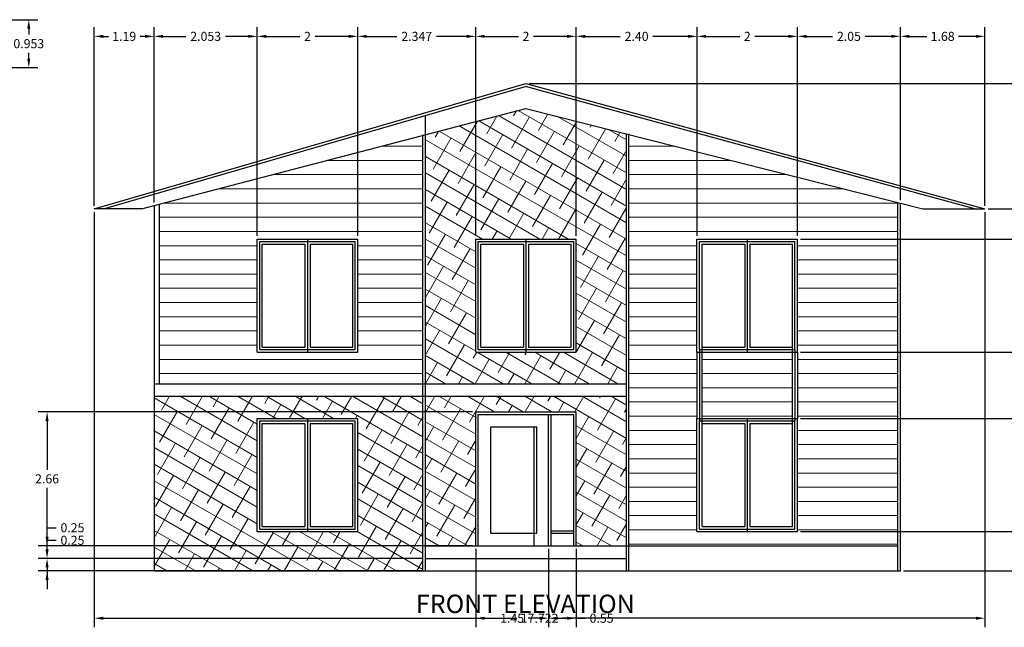
# Model space of a CAD drawing. Units: metres. Extents: x 14054 to 28215, y 4175 to 8383.
# Tile 4 of 6: x 14077.36 to 14096.96, y 4179.61 to 4191.69. Entities that reach past the tile are written whole.
import ezdxf

# ---------------------------------------------------------------- set-up
doc = ezdxf.new("R2010")
doc.units = ezdxf.units.M
for name, color, linetype, lineweight in [('A-ANNO-DIMS', 2, 'Continuous', 18), ('A-ANNO-TEXT', 3, 'Continuous', 18), ('A-ELEV', 7, 'Continuous', 25), ('A-WALL-PATT', 8, 'Continuous', 13)]:
    doc.layers.add(name, color=color, linetype=linetype, lineweight=lineweight)
doc.styles.get("Standard").update_dxf_attribs({"font": 'arial.ttf'})
doc.dimstyles.get("Standard").update_dxf_attribs({"dimtxt": 0.18, "dimasz": 0.18, "dimexe": 0.18, "dimexo": 0.0625, "dimgap": 0.09, "dimtad": 0, "dimtih": 1, "dimtoh": 1, "dimdec": 4, "dimzin": 0, "dimdsep": 46, "dimtxsty": 'Standard', "dimcen": 0.09, "dimadec": 0, "dimazin": 0, "dimtfac": 1, "dimtdec": 4, "dimtofl": 0, "dimtmove": 0, "dimatfit": 3, "dimfxl": 1, "dimtolj": 1, "dimtzin": 0, "dimarcsym": 0})

# ---------------------------------------------------------------- blocks, each defined once
blk = doc.blocks.new('*D13')
at = {"layer": 'A-ANNO-DIMS', "color": 0, "lineweight": -2, "transparency": 16777216}
for p, q in [((14078.849, 4187.865), (14078.849, 4179.608)), ((14096.571, 4187.865), (14096.571, 4179.608)), ((14079.029, 4179.788), (14087.256, 4179.788)), ((14096.391, 4179.788), (14088.164, 4179.788))]:
    blk.add_line(p, q, dxfattribs=at)
at = {"layer": 'A-ANNO-DIMS', "color": 0, "transparency": 16777216}
for points in [[(14079.029, 4179.818), (14079.029, 4179.758), (14078.849, 4179.788)], [(14096.391, 4179.818), (14096.391, 4179.758), (14096.571, 4179.788)]]:
    blk.add_solid(points, dxfattribs=at)
at = {"layer": 'Defpoints', "color": 0, "transparency": 16777216}
for p in [(14078.849, 4187.928), (14096.571, 4187.928), (14096.571, 4179.788)]:
    blk.add_point(p, dxfattribs=at)
at = {"layer": 'A-ANNO-DIMS', "color": 0, "transparency": 16777216, "insert": (14087.71, 4179.788), "char_height": 0.18, "attachment_point": 5}
blk.add_mtext('\\A1;17.722', dxfattribs=at)
blk = doc.blocks.new('*D14')
at = {"layer": 'A-ANNO-DIMS', "color": 0, "lineweight": -2, "transparency": 16777216}
for p, q in [((14078.849, 4187.99), (14078.849, 4191.54)), ((14080.038, 4188.055), (14080.038, 4191.54)), ((14079.029, 4191.36), (14079.128, 4191.36)), ((14079.858, 4191.36), (14079.759, 4191.36))]:
    blk.add_line(p, q, dxfattribs=at)
at = {"layer": 'A-ANNO-DIMS', "color": 0, "transparency": 16777216}
for points in [[(14079.029, 4191.39), (14079.029, 4191.33), (14078.849, 4191.36)], [(14079.858, 4191.39), (14079.858, 4191.33), (14080.038, 4191.36)]]:
    blk.add_solid(points, dxfattribs=at)
at = {"layer": 'Defpoints', "color": 0, "transparency": 16777216}
for p in [(14080.038, 4191.36), (14078.849, 4187.928), (14080.038, 4187.993)]:
    blk.add_point(p, dxfattribs=at)
at = {"layer": 'A-ANNO-DIMS', "color": 0, "transparency": 16777216, "insert": (14079.444, 4191.36), "char_height": 0.18, "attachment_point": 5}
blk.add_mtext('\\A1;1.19', dxfattribs=at)
blk = doc.blocks.new('*D15')
at = {"layer": 'A-ANNO-DIMS', "color": 0, "lineweight": -2, "transparency": 16777216}
for p, q in [((14080.038, 4188.055), (14080.038, 4191.54)), ((14082.091, 4187.392), (14082.091, 4191.54)), ((14080.218, 4191.36), (14080.669, 4191.36)), ((14081.911, 4191.36), (14081.46, 4191.36))]:
    blk.add_line(p, q, dxfattribs=at)
at = {"layer": 'A-ANNO-DIMS', "color": 0, "transparency": 16777216}
for points in [[(14080.218, 4191.39), (14080.218, 4191.33), (14080.038, 4191.36)], [(14081.911, 4191.39), (14081.911, 4191.33), (14082.091, 4191.36)]]:
    blk.add_solid(points, dxfattribs=at)
at = {"layer": 'Defpoints', "color": 0, "transparency": 16777216}
for p in [(14082.091, 4191.36), (14080.038, 4187.993), (14082.091, 4187.329)]:
    blk.add_point(p, dxfattribs=at)
at = {"layer": 'A-ANNO-DIMS', "color": 0, "transparency": 16777216, "insert": (14081.065, 4191.36), "char_height": 0.18, "attachment_point": 5}
blk.add_mtext('\\A1;2.053', dxfattribs=at)
blk = doc.blocks.new('*D16')
at = {"layer": 'A-ANNO-DIMS', "color": 0, "lineweight": -2, "transparency": 16777216}
for p, q in [((14082.091, 4187.392), (14082.091, 4191.54)), ((14084.091, 4187.392), (14084.091, 4191.54)), ((14082.271, 4191.36), (14082.941, 4191.36)), ((14083.911, 4191.36), (14083.241, 4191.36))]:
    blk.add_line(p, q, dxfattribs=at)
at = {"layer": 'A-ANNO-DIMS', "color": 0, "transparency": 16777216}
for points in [[(14082.271, 4191.39), (14082.271, 4191.33), (14082.091, 4191.36)], [(14083.911, 4191.39), (14083.911, 4191.33), (14084.091, 4191.36)]]:
    blk.add_solid(points, dxfattribs=at)
at = {"layer": 'Defpoints', "color": 0, "transparency": 16777216}
for p in [(14084.091, 4191.36), (14082.091, 4187.329), (14084.091, 4187.329)]:
    blk.add_point(p, dxfattribs=at)
at = {"layer": 'A-ANNO-DIMS', "color": 0, "transparency": 16777216, "insert": (14083.091, 4191.36), "char_height": 0.18, "attachment_point": 5}
blk.add_mtext('\\A1;2', dxfattribs=at)
blk = doc.blocks.new('*D17')
at = {"layer": 'A-ANNO-DIMS', "color": 0, "lineweight": -2, "transparency": 16777216}
for p, q in [((14084.091, 4187.392), (14084.091, 4191.54)), ((14086.438, 4187.392), (14086.438, 4191.54)), ((14084.271, 4191.36), (14084.869, 4191.36)), ((14086.258, 4191.36), (14085.66, 4191.36))]:
    blk.add_line(p, q, dxfattribs=at)
at = {"layer": 'A-ANNO-DIMS', "color": 0, "transparency": 16777216}
for points in [[(14084.271, 4191.39), (14084.271, 4191.33), (14084.091, 4191.36)], [(14086.258, 4191.39), (14086.258, 4191.33), (14086.438, 4191.36)]]:
    blk.add_solid(points, dxfattribs=at)
at = {"layer": 'Defpoints', "color": 0, "transparency": 16777216}
for p in [(14086.438, 4191.36), (14084.091, 4187.329), (14086.438, 4187.329)]:
    blk.add_point(p, dxfattribs=at)
at = {"layer": 'A-ANNO-DIMS', "color": 0, "transparency": 16777216, "insert": (14085.265, 4191.36), "char_height": 0.18, "attachment_point": 5}
blk.add_mtext('\\A1;2.347', dxfattribs=at)
blk = doc.blocks.new('*D18')
at = {"layer": 'A-ANNO-DIMS', "color": 0, "lineweight": -2, "transparency": 16777216}
for p, q in [((14086.438, 4187.392), (14086.438, 4191.54)), ((14088.438, 4187.392), (14088.438, 4191.54)), ((14086.618, 4191.36), (14087.289, 4191.36)), ((14088.258, 4191.36), (14087.588, 4191.36))]:
    blk.add_line(p, q, dxfattribs=at)
at = {"layer": 'A-ANNO-DIMS', "color": 0, "transparency": 16777216}
for points in [[(14086.618, 4191.39), (14086.618, 4191.33), (14086.438, 4191.36)], [(14088.258, 4191.39), (14088.258, 4191.33), (14088.438, 4191.36)]]:
    blk.add_solid(points, dxfattribs=at)
at = {"layer": 'Defpoints', "color": 0, "transparency": 16777216}
for p in [(14088.438, 4191.36), (14086.438, 4187.329), (14088.438, 4187.329)]:
    blk.add_point(p, dxfattribs=at)
at = {"layer": 'A-ANNO-DIMS', "color": 0, "transparency": 16777216, "insert": (14087.438, 4191.36), "char_height": 0.18, "attachment_point": 5}
blk.add_mtext('\\A1;2', dxfattribs=at)
blk = doc.blocks.new('*D19')
at = {"layer": 'A-ANNO-DIMS', "color": 0, "lineweight": -2, "transparency": 16777216}
for p, q in [((14088.438, 4187.392), (14088.438, 4191.54)), ((14090.842, 4187.392), (14090.842, 4191.54)), ((14088.618, 4191.36), (14089.315, 4191.36)), ((14090.662, 4191.36), (14089.965, 4191.36))]:
    blk.add_line(p, q, dxfattribs=at)
at = {"layer": 'A-ANNO-DIMS', "color": 0, "transparency": 16777216}
for points in [[(14088.618, 4191.39), (14088.618, 4191.33), (14088.438, 4191.36)], [(14090.662, 4191.39), (14090.662, 4191.33), (14090.842, 4191.36)]]:
    blk.add_solid(points, dxfattribs=at)
at = {"layer": 'Defpoints', "color": 0, "transparency": 16777216}
for p in [(14090.842, 4191.36), (14088.438, 4187.329), (14090.842, 4187.329)]:
    blk.add_point(p, dxfattribs=at)
at = {"layer": 'A-ANNO-DIMS', "color": 0, "transparency": 16777216, "insert": (14089.64, 4191.36), "char_height": 0.18, "attachment_point": 5}
blk.add_mtext('\\A1;2.40', dxfattribs=at)
blk = doc.blocks.new('*D20')
at = {"layer": 'A-ANNO-DIMS', "color": 0, "lineweight": -2, "transparency": 16777216}
for p, q in [((14090.842, 4187.392), (14090.842, 4191.54)), ((14092.842, 4187.392), (14092.842, 4191.54)), ((14091.022, 4191.36), (14091.692, 4191.36)), ((14092.662, 4191.36), (14091.991, 4191.36))]:
    blk.add_line(p, q, dxfattribs=at)
at = {"layer": 'A-ANNO-DIMS', "color": 0, "transparency": 16777216}
for points in [[(14091.022, 4191.39), (14091.022, 4191.33), (14090.842, 4191.36)], [(14092.662, 4191.39), (14092.662, 4191.33), (14092.842, 4191.36)]]:
    blk.add_solid(points, dxfattribs=at)
at = {"layer": 'Defpoints', "color": 0, "transparency": 16777216}
for p in [(14092.842, 4191.36), (14090.842, 4187.329), (14092.842, 4187.329)]:
    blk.add_point(p, dxfattribs=at)
at = {"layer": 'A-ANNO-DIMS', "color": 0, "transparency": 16777216, "insert": (14091.842, 4191.36), "char_height": 0.18, "attachment_point": 5}
blk.add_mtext('\\A1;2', dxfattribs=at)
blk = doc.blocks.new('*D21')
at = {"layer": 'A-ANNO-DIMS', "color": 0, "lineweight": -2, "transparency": 16777216}
for p, q in [((14092.842, 4187.392), (14092.842, 4191.54)), ((14094.888, 4188.104), (14094.888, 4191.54)), ((14093.022, 4191.36), (14093.539, 4191.36)), ((14094.708, 4191.36), (14094.191, 4191.36))]:
    blk.add_line(p, q, dxfattribs=at)
at = {"layer": 'A-ANNO-DIMS', "color": 0, "transparency": 16777216}
for points in [[(14093.022, 4191.39), (14093.022, 4191.33), (14092.842, 4191.36)], [(14094.708, 4191.39), (14094.708, 4191.33), (14094.888, 4191.36)]]:
    blk.add_solid(points, dxfattribs=at)
at = {"layer": 'Defpoints', "color": 0, "transparency": 16777216}
for p in [(14094.888, 4191.36), (14094.888, 4188.041), (14092.842, 4187.329)]:
    blk.add_point(p, dxfattribs=at)
at = {"layer": 'A-ANNO-DIMS', "color": 0, "transparency": 16777216, "insert": (14093.865, 4191.36), "char_height": 0.18, "attachment_point": 5}
blk.add_mtext('\\A1;2.05', dxfattribs=at)
blk = doc.blocks.new('*D22')
at = {"layer": 'A-ANNO-DIMS', "color": 0, "lineweight": -2, "transparency": 16777216}
for p, q in [((14094.888, 4188.104), (14094.888, 4191.54)), ((14096.571, 4187.99), (14096.571, 4191.54)), ((14095.068, 4191.36), (14095.414, 4191.36)), ((14096.391, 4191.36), (14096.045, 4191.36))]:
    blk.add_line(p, q, dxfattribs=at)
at = {"layer": 'A-ANNO-DIMS', "color": 0, "transparency": 16777216}
for points in [[(14095.068, 4191.39), (14095.068, 4191.33), (14094.888, 4191.36)], [(14096.391, 4191.39), (14096.391, 4191.33), (14096.571, 4191.36)]]:
    blk.add_solid(points, dxfattribs=at)
at = {"layer": 'Defpoints', "color": 0, "transparency": 16777216}
for p in [(14096.571, 4191.36), (14094.888, 4188.041), (14096.571, 4187.928)]:
    blk.add_point(p, dxfattribs=at)
at = {"layer": 'A-ANNO-DIMS', "color": 0, "transparency": 16777216, "insert": (14095.73, 4191.36), "char_height": 0.18, "attachment_point": 5}
blk.add_mtext('\\A1;1.68', dxfattribs=at)
blk = doc.blocks.new('*D23')
at = {"layer": 'A-ANNO-DIMS', "color": 0, "lineweight": -2, "transparency": 16777216}
for p, q in [((14097.511, 4181.511), (14097.511, 4181.691)), ((14097.511, 4181.691), (14097.691, 4181.691)), ((14092.904, 4181.511), (14097.691, 4181.511)), ((14097.511, 4180.908), (14097.511, 4181.331)), ((14094.951, 4180.728), (14097.691, 4180.728))]:
    blk.add_line(p, q, dxfattribs=at)
at = {"layer": 'A-ANNO-DIMS', "color": 0, "transparency": 16777216}
for points in [[(14097.481, 4181.331), (14097.541, 4181.331), (14097.511, 4181.511)], [(14097.481, 4180.908), (14097.541, 4180.908), (14097.511, 4180.728)]]:
    blk.add_solid(points, dxfattribs=at)
at = {"layer": 'Defpoints', "color": 0, "transparency": 16777216}
for p in [(14092.842, 4181.511), (14097.511, 4181.511), (14094.888, 4180.728)]:
    blk.add_point(p, dxfattribs=at)
at = {"layer": 'A-ANNO-DIMS', "color": 0, "transparency": 16777216, "insert": (14098.084, 4181.691), "char_height": 0.18, "attachment_point": 5}
blk.add_mtext('\\A1;0.784', dxfattribs=at)
blk = doc.blocks.new('*D24')
at = {"layer": 'A-ANNO-DIMS', "color": 0, "lineweight": -2, "transparency": 16777216}
for p, q in [((14092.904, 4183.761), (14097.691, 4183.761)), ((14097.511, 4183.581), (14097.511, 4182.818)), ((14097.511, 4181.691), (14097.511, 4182.454)), ((14092.904, 4181.511), (14097.691, 4181.511))]:
    blk.add_line(p, q, dxfattribs=at)
at = {"layer": 'A-ANNO-DIMS', "color": 0, "transparency": 16777216}
for points in [[(14097.481, 4183.581), (14097.541, 4183.581), (14097.511, 4183.761)], [(14097.481, 4181.691), (14097.541, 4181.691), (14097.511, 4181.511)]]:
    blk.add_solid(points, dxfattribs=at)
at = {"layer": 'Defpoints', "color": 0, "transparency": 16777216}
for p in [(14092.842, 4183.761), (14097.511, 4183.761), (14092.842, 4181.511)]:
    blk.add_point(p, dxfattribs=at)
at = {"layer": 'A-ANNO-DIMS', "color": 0, "transparency": 16777216, "insert": (14097.511, 4182.636), "char_height": 0.18, "attachment_point": 5}
blk.add_mtext('\\A1;2.25', dxfattribs=at)
blk = doc.blocks.new('*D25')
at = {"layer": 'A-ANNO-DIMS', "color": 0, "lineweight": -2, "transparency": 16777216}
for p, q in [((14092.904, 4185.079), (14097.691, 4185.079)), ((14097.511, 4184.899), (14097.511, 4184.602)), ((14097.511, 4183.941), (14097.511, 4184.238)), ((14092.904, 4183.761), (14097.691, 4183.761))]:
    blk.add_line(p, q, dxfattribs=at)
at = {"layer": 'A-ANNO-DIMS', "color": 0, "transparency": 16777216}
for points in [[(14097.481, 4184.899), (14097.541, 4184.899), (14097.511, 4185.079)], [(14097.481, 4183.941), (14097.541, 4183.941), (14097.511, 4183.761)]]:
    blk.add_solid(points, dxfattribs=at)
at = {"layer": 'Defpoints', "color": 0, "transparency": 16777216}
for p in [(14092.842, 4185.079), (14097.511, 4185.079), (14092.842, 4183.761)]:
    blk.add_point(p, dxfattribs=at)
at = {"layer": 'A-ANNO-DIMS', "color": 0, "transparency": 16777216, "insert": (14097.511, 4184.42), "char_height": 0.18, "attachment_point": 5}
blk.add_mtext('\\A1;1.318', dxfattribs=at)
blk = doc.blocks.new('*D26')
at = {"layer": 'A-ANNO-DIMS', "color": 0, "lineweight": -2, "transparency": 16777216}
for p, q in [((14092.904, 4187.329), (14097.691, 4187.329)), ((14097.511, 4187.149), (14097.511, 4186.386)), ((14097.511, 4185.259), (14097.511, 4186.022)), ((14092.904, 4185.079), (14097.691, 4185.079))]:
    blk.add_line(p, q, dxfattribs=at)
at = {"layer": 'A-ANNO-DIMS', "color": 0, "transparency": 16777216}
for points in [[(14097.481, 4187.149), (14097.541, 4187.149), (14097.511, 4187.329)], [(14097.481, 4185.259), (14097.541, 4185.259), (14097.511, 4185.079)]]:
    blk.add_solid(points, dxfattribs=at)
at = {"layer": 'Defpoints', "color": 0, "transparency": 16777216}
for p in [(14092.842, 4187.329), (14097.511, 4187.329), (14092.842, 4185.079)]:
    blk.add_point(p, dxfattribs=at)
at = {"layer": 'A-ANNO-DIMS', "color": 0, "transparency": 16777216, "insert": (14097.511, 4186.204), "char_height": 0.18, "attachment_point": 5}
blk.add_mtext('\\A1;2.25', dxfattribs=at)
blk = doc.blocks.new('*D27')
at = {"layer": 'A-ANNO-DIMS', "color": 0, "lineweight": -2, "transparency": 16777216}
for p, q in [((14097.511, 4187.928), (14097.511, 4188.108)), ((14097.511, 4188.108), (14097.691, 4188.108)), ((14096.633, 4187.928), (14097.691, 4187.928)), ((14097.511, 4187.509), (14097.511, 4187.748)), ((14092.904, 4187.329), (14097.691, 4187.329))]:
    blk.add_line(p, q, dxfattribs=at)
at = {"layer": 'A-ANNO-DIMS', "color": 0, "transparency": 16777216}
for points in [[(14097.481, 4187.748), (14097.541, 4187.748), (14097.511, 4187.928)], [(14097.481, 4187.509), (14097.541, 4187.509), (14097.511, 4187.329)]]:
    blk.add_solid(points, dxfattribs=at)
at = {"layer": 'Defpoints', "color": 0, "transparency": 16777216}
for p in [(14096.571, 4187.928), (14097.511, 4187.928), (14092.842, 4187.329)]:
    blk.add_point(p, dxfattribs=at)
at = {"layer": 'A-ANNO-DIMS', "color": 0, "transparency": 16777216, "insert": (14098.014, 4188.108), "char_height": 0.18, "attachment_point": 5}
blk.add_mtext('\\A1;0.60', dxfattribs=at)
blk = doc.blocks.new('*D28')
at = {"layer": 'A-ANNO-DIMS', "color": 0, "lineweight": -2, "transparency": 16777216}
for p, q in [((14087.501, 4190.42), (14097.691, 4190.42)), ((14097.511, 4190.24), (14097.511, 4189.356)), ((14097.511, 4188.108), (14097.511, 4188.992)), ((14096.633, 4187.928), (14097.691, 4187.928))]:
    blk.add_line(p, q, dxfattribs=at)
at = {"layer": 'A-ANNO-DIMS', "color": 0, "transparency": 16777216}
for points in [[(14097.481, 4190.24), (14097.541, 4190.24), (14097.511, 4190.42)], [(14097.481, 4188.108), (14097.541, 4188.108), (14097.511, 4187.928)]]:
    blk.add_solid(points, dxfattribs=at)
at = {"layer": 'Defpoints', "color": 0, "transparency": 16777216}
for p in [(14087.438, 4190.42), (14097.511, 4190.42), (14096.571, 4187.928)]:
    blk.add_point(p, dxfattribs=at)
at = {"layer": 'A-ANNO-DIMS', "color": 0, "transparency": 16777216, "insert": (14097.511, 4189.174), "char_height": 0.18, "attachment_point": 5}
blk.add_mtext('\\A1;2.49', dxfattribs=at)
blk = doc.blocks.new('*D40')
at = {"layer": 'A-ANNO-DIMS', "color": 0, "lineweight": -2, "transparency": 16777216}
for p, q in [((14086.438, 4181.165), (14086.438, 4179.608)), ((14087.888, 4181.165), (14087.888, 4179.608)), ((14086.618, 4179.788), (14086.847, 4179.788)), ((14087.708, 4179.788), (14087.479, 4179.788))]:
    blk.add_line(p, q, dxfattribs=at)
at = {"layer": 'A-ANNO-DIMS', "color": 0, "transparency": 16777216}
for points in [[(14086.618, 4179.818), (14086.618, 4179.758), (14086.438, 4179.788)], [(14087.708, 4179.818), (14087.708, 4179.758), (14087.888, 4179.788)]]:
    blk.add_solid(points, dxfattribs=at)
at = {"layer": 'Defpoints', "color": 0, "transparency": 16777216}
for p in [(14086.438, 4181.228), (14087.888, 4181.228), (14087.888, 4179.788)]:
    blk.add_point(p, dxfattribs=at)
at = {"layer": 'A-ANNO-DIMS', "color": 0, "transparency": 16777216, "insert": (14087.163, 4179.788), "char_height": 0.18, "attachment_point": 5}
blk.add_mtext('\\A1;1.45', dxfattribs=at)
blk = doc.blocks.new('*D41')
at = {"layer": 'A-ANNO-DIMS', "color": 0, "lineweight": -2, "transparency": 16777216}
for p, q in [((14087.888, 4181.165), (14087.888, 4179.608)), ((14088.438, 4181.165), (14088.438, 4179.608)), ((14088.068, 4179.788), (14088.258, 4179.788)), ((14088.438, 4179.788), (14088.618, 4179.788))]:
    blk.add_line(p, q, dxfattribs=at)
at = {"layer": 'A-ANNO-DIMS', "color": 0, "transparency": 16777216}
for points in [[(14088.068, 4179.818), (14088.068, 4179.758), (14087.888, 4179.788)], [(14088.258, 4179.818), (14088.258, 4179.758), (14088.438, 4179.788)]]:
    blk.add_solid(points, dxfattribs=at)
at = {"layer": 'Defpoints', "color": 0, "transparency": 16777216}
for p in [(14087.888, 4181.228), (14088.438, 4181.228), (14088.438, 4179.788)]:
    blk.add_point(p, dxfattribs=at)
at = {"layer": 'A-ANNO-DIMS', "color": 0, "transparency": 16777216, "insert": (14088.943, 4179.788), "char_height": 0.18, "attachment_point": 5}
blk.add_mtext('\\A1;0.55', dxfattribs=at)
blk = doc.blocks.new('*D42')
at = {"layer": 'A-ANNO-DIMS', "color": 0, "lineweight": -2, "transparency": 16777216}
for p, q in [((14086.376, 4183.892), (14077.729, 4183.892)), ((14077.909, 4183.712), (14077.909, 4182.742)), ((14077.909, 4181.408), (14077.909, 4182.378)), ((14086.376, 4181.228), (14077.729, 4181.228))]:
    blk.add_line(p, q, dxfattribs=at)
at = {"layer": 'A-ANNO-DIMS', "color": 0, "transparency": 16777216}
for points in [[(14077.879, 4183.712), (14077.939, 4183.712), (14077.909, 4183.892)], [(14077.879, 4181.408), (14077.939, 4181.408), (14077.909, 4181.228)]]:
    blk.add_solid(points, dxfattribs=at)
at = {"layer": 'Defpoints', "color": 0, "transparency": 16777216}
for p in [(14077.909, 4183.892), (14086.438, 4183.892), (14086.438, 4181.228)]:
    blk.add_point(p, dxfattribs=at)
at = {"layer": 'A-ANNO-DIMS', "color": 0, "transparency": 16777216, "insert": (14077.909, 4182.56), "char_height": 0.18, "attachment_point": 5}
blk.add_mtext('\\A1;2.66', dxfattribs=at)
blk = doc.blocks.new('*D43')
at = {"layer": 'A-ANNO-DIMS', "color": 0, "lineweight": -2, "transparency": 16777216}
for p, q in [((14077.909, 4181.158), (14077.909, 4181.338)), ((14077.909, 4181.338), (14078.089, 4181.338)), ((14085.376, 4180.978), (14077.729, 4180.978)), ((14085.376, 4180.728), (14077.729, 4180.728)), ((14077.909, 4180.548), (14077.909, 4180.368))]:
    blk.add_line(p, q, dxfattribs=at)
at = {"layer": 'A-ANNO-DIMS', "color": 0, "transparency": 16777216}
for points in [[(14077.879, 4181.158), (14077.939, 4181.158), (14077.909, 4180.978)], [(14077.879, 4180.548), (14077.939, 4180.548), (14077.909, 4180.728)]]:
    blk.add_solid(points, dxfattribs=at)
at = {"layer": 'Defpoints', "color": 0, "transparency": 16777216}
for p in [(14077.909, 4180.978), (14085.438, 4180.978), (14085.438, 4180.728)]:
    blk.add_point(p, dxfattribs=at)
at = {"layer": 'A-ANNO-DIMS', "color": 0, "transparency": 16777216, "insert": (14078.414, 4181.338), "char_height": 0.18, "attachment_point": 5}
blk.add_mtext('\\A1;0.25', dxfattribs=at)
blk = doc.blocks.new('*D44')
at = {"layer": 'A-ANNO-DIMS', "color": 0, "lineweight": -2, "transparency": 16777216}
for p, q in [((14077.909, 4181.408), (14077.909, 4181.588)), ((14077.909, 4181.588), (14078.089, 4181.588)), ((14085.376, 4181.228), (14077.729, 4181.228)), ((14085.376, 4180.978), (14077.729, 4180.978)), ((14077.909, 4180.798), (14077.909, 4180.618))]:
    blk.add_line(p, q, dxfattribs=at)
at = {"layer": 'A-ANNO-DIMS', "color": 0, "transparency": 16777216}
for points in [[(14077.879, 4181.408), (14077.939, 4181.408), (14077.909, 4181.228)], [(14077.879, 4180.798), (14077.939, 4180.798), (14077.909, 4180.978)]]:
    blk.add_solid(points, dxfattribs=at)
at = {"layer": 'Defpoints', "color": 0, "transparency": 16777216}
for p in [(14077.909, 4181.228), (14085.438, 4181.228), (14085.438, 4180.978)]:
    blk.add_point(p, dxfattribs=at)
at = {"layer": 'A-ANNO-DIMS', "color": 0, "transparency": 16777216, "insert": (14078.414, 4181.588), "char_height": 0.18, "attachment_point": 5}
blk.add_mtext('\\A1;0.25', dxfattribs=at)
blk = doc.blocks.new('*D75')
at = {"layer": 'A-ANNO-DIMS', "color": 0, "lineweight": -2, "transparency": 16777216}
for p, q in [((14073.161, 4191.691), (14077.725, 4191.691)), ((14077.545, 4191.511), (14077.545, 4191.397)), ((14077.545, 4190.918), (14077.545, 4191.033)), ((14073.161, 4190.738), (14077.725, 4190.738))]:
    blk.add_line(p, q, dxfattribs=at)
at = {"layer": 'A-ANNO-DIMS', "color": 0, "transparency": 16777216}
for points in [[(14077.515, 4191.511), (14077.575, 4191.511), (14077.545, 4191.691)], [(14077.515, 4190.918), (14077.575, 4190.918), (14077.545, 4190.738)]]:
    blk.add_solid(points, dxfattribs=at)
at = {"layer": 'Defpoints', "color": 0, "transparency": 16777216}
for p in [(14073.099, 4191.691), (14073.099, 4190.738), (14077.545, 4190.738)]:
    blk.add_point(p, dxfattribs=at)
at = {"layer": 'A-ANNO-DIMS', "color": 0, "transparency": 16777216, "insert": (14077.545, 4191.215), "char_height": 0.18, "attachment_point": 5}
blk.add_mtext('\\A1;0.953', dxfattribs=at)

msp = doc.modelspace()

# ---------------------------------------------------------------- hatches: boundary and pattern name
at = {"layer": 'A-WALL-PATT'}
h = msp.add_hatch(dxfattribs=at)
h.set_pattern_fill('ANSI38', color=256, scale=0.09, angle=105)
h.paths.add_polyline_path([(14085.3882, 4184.2025), (14080.0382, 4184.2025), (14080.0382, 4180.7275), (14085.3882, 4180.7275)])
h.paths.add_polyline_path([(14084.091, 4183.7614), (14084.091, 4181.5114), (14082.091, 4181.5114), (14082.091, 4183.7614)], flags=16)
h.paths.add_polyline_path([(14084.041, 4183.7114), (14084.041, 4181.5614), (14082.141, 4181.5614), (14082.141, 4183.7114)], flags=0)
h.paths.add_polyline_path([(14083.991, 4183.6614), (14083.991, 4181.6114), (14083.141, 4181.6114), (14083.141, 4183.6614)], flags=0)
h.paths.add_polyline_path([(14083.041, 4183.6614), (14083.041, 4181.6114), (14082.191, 4181.6114), (14082.191, 4183.6614)], flags=0)
h.paths.add_polyline_path([(14086.4382, 4183.892), (14088.4382, 4183.892), (14088.4382, 4181.2275), (14089.4382, 4181.2275), (14089.4382, 4184.2025), (14085.4382, 4184.2025), (14085.4382, 4181.2275), (14086.4382, 4181.2275)])
h.paths.add_polyline_path([(14089.4382, 4189.4203), (14087.4382, 4189.9263), (14085.4382, 4189.4038), (14085.4382, 4184.4525), (14089.4382, 4184.4525)])
h.paths.add_polyline_path([(14086.4382, 4187.3294), (14088.4382, 4187.3294), (14088.4382, 4185.0794), (14086.4382, 4185.0794)], flags=16)
h.paths.add_polyline_path([(14086.4882, 4187.2794), (14088.3882, 4187.2794), (14088.3882, 4185.1294), (14086.4882, 4185.1294)], flags=0)
h.paths.add_polyline_path([(14086.5382, 4187.2294), (14087.3882, 4187.2294), (14087.3882, 4185.1794), (14086.5382, 4185.1794)], flags=0)
h.paths.add_polyline_path([(14087.4882, 4187.2294), (14088.3382, 4187.2294), (14088.3382, 4185.1794), (14087.4882, 4185.1794)], flags=0)
h = msp.add_hatch(dxfattribs=at)
h.set_pattern_fill('ANSI31', color=256, scale=0.089, angle=135)
h.paths.add_polyline_path([(14085.3882, 4189.3907), (14080.1382, 4188.019), (14080.1382, 4184.4525), (14085.3882, 4184.4525)])
h.paths.add_polyline_path([(14084.091, 4187.3294), (14084.091, 4185.0794), (14082.091, 4185.0794), (14082.091, 4187.3294)], flags=16)
h.paths.add_polyline_path([(14084.041, 4187.2794), (14084.041, 4185.1294), (14082.141, 4185.1294), (14082.141, 4187.2794)], flags=0)
h.paths.add_polyline_path([(14083.991, 4187.2294), (14083.991, 4185.1794), (14083.141, 4185.1794), (14083.141, 4187.2294)], flags=0)
h.paths.add_polyline_path([(14083.041, 4187.2294), (14083.041, 4185.1794), (14082.191, 4185.1794), (14082.191, 4187.2294)], flags=0)
h = msp.add_hatch(dxfattribs=at)
h.set_pattern_fill('ANSI31', color=256, scale=0.089, angle=135)
h.paths.add_polyline_path([(14094.8382, 4188.054), (14089.4882, 4189.4077), (14089.4882, 4181.2275), (14094.8382, 4181.2275)])
h.paths.add_polyline_path([(14090.8417, 4187.3294), (14092.8417, 4187.3294), (14092.8417, 4185.0794), (14092.8417, 4183.7614), (14092.8417, 4181.5114), (14090.8417, 4181.5114), (14090.8417, 4183.7614), (14090.8417, 4185.0794)], flags=16)
h.paths.add_polyline_path([(14090.8917, 4187.2794), (14092.7917, 4187.2794), (14092.7917, 4185.1294), (14092.7917, 4183.7114), (14092.7917, 4181.5614), (14090.8917, 4181.5614), (14090.8917, 4183.7114), (14090.8917, 4185.1294)], flags=0)
h.paths.add_polyline_path([(14090.9417, 4187.2294), (14091.7917, 4187.2294), (14091.7917, 4185.1794), (14090.9417, 4185.1794), (14090.9417, 4185.1294), (14092.7417, 4185.1294), (14092.7417, 4185.1794), (14091.8917, 4185.1794), (14091.8917, 4187.2294), (14092.7417, 4187.2294), (14092.7417, 4185.1794), (14092.7417, 4183.6614), (14092.7417, 4181.6114), (14091.8917, 4181.6114), (14091.8917, 4183.6614), (14092.7417, 4183.6614), (14092.7417, 4183.7114), (14090.9417, 4183.7114), (14090.9417, 4183.6614), (14091.7917, 4183.6614), (14091.7917, 4181.6114), (14090.9417, 4181.6114), (14090.9417, 4183.6614), (14090.9417, 4185.1794)], flags=0)
h = msp.add_hatch(dxfattribs=at)
h.set_pattern_fill('ANSI31', color=256, scale=0.089, angle=135)
h.paths.add_polyline_path([(14092.7417, 4185.0794), (14090.9417, 4185.0794), (14090.9417, 4183.7614), (14092.7417, 4183.7614)])

# ---------------------------------------------------------------- linework, layer by layer
at = {"layer": 'A-ELEV'}
for p, q in [((14078.8491, 4187.9275), (14087.4382, 4190.4202)), ((14079.0285, 4187.9275), (14087.4522, 4190.3722)), ((14087.425, 4190.372), (14096.3811, 4187.9275)), ((14087.4382, 4190.4202), (14096.571, 4187.9275)), ((14079.7882, 4187.9275), (14087.4382, 4189.9263)), ((14085.4382, 4184.2025), (14085.4382, 4189.7877)), ((14087.4382, 4189.9263), (14095.3382, 4187.9275)), ((14085.3882, 4184.2025), (14085.3882, 4189.4038)), ((14089.4382, 4180.7275), (14089.4382, 4189.4203)), ((14089.4882, 4180.7275), (14089.4882, 4189.4203)), ((14080.1382, 4188.019), (14080.1382, 4184.4525)), ((14094.8382, 4180.7275), (14094.8382, 4188.054)), ((14094.8882, 4180.7275), (14094.8882, 4188.0414)), ((14079.7882, 4187.9275), (14078.8491, 4187.9275)), ((14080.0382, 4187.9928), (14080.0382, 4180.7275)), ((14095.3382, 4187.9275), (14096.571, 4187.9275)), ((14082.091, 4185.0794), (14082.091, 4187.3294)), ((14082.091, 4187.3294), (14084.091, 4187.3294)), ((14082.141, 4187.2794), (14084.041, 4187.2794)), ((14082.141, 4185.1294), (14082.141, 4187.2794)), ((14082.191, 4187.2294), (14083.041, 4187.2294)), ((14082.191, 4185.1794), (14082.191, 4187.2294)), ((14083.041, 4187.2294), (14083.041, 4185.1794)), ((14083.091, 4187.3294), (14083.091, 4185.0794)), ((14083.141, 4187.2294), (14083.991, 4187.2294)), ((14083.141, 4187.2294), (14083.141, 4185.1794)), ((14083.991, 4185.1794), (14083.991, 4187.2294)), ((14084.041, 4185.1294), (14084.041, 4187.2794)), ((14084.091, 4185.0794), (14084.091, 4187.3294)), ((14086.4382, 4185.0794), (14086.4382, 4187.3294)), ((14086.4382, 4187.3294), (14088.4382, 4187.3294)), ((14086.4882, 4185.1294), (14086.4882, 4187.2794)), ((14086.4882, 4187.2794), (14088.3882, 4187.2794)), ((14086.5382, 4185.1794), (14086.5382, 4187.2294)), ((14086.5382, 4187.2294), (14087.3882, 4187.2294)), ((14087.3882, 4187.2294), (14087.3882, 4185.1794)), ((14087.4382, 4187.3294), (14087.4382, 4185.0794)), ((14087.4882, 4187.2294), (14088.3382, 4187.2294)), ((14087.4882, 4187.2294), (14087.4882, 4185.1794)), ((14088.3382, 4185.1794), (14088.3382, 4187.2294)), ((14088.3882, 4185.1294), (14088.3882, 4187.2794)), ((14088.4382, 4185.0794), (14088.4382, 4187.3294)), ((14090.8417, 4185.0794), (14090.8417, 4187.3294)), ((14090.8417, 4187.3294), (14092.8417, 4187.3294)), ((14090.8917, 4185.1294), (14090.8917, 4187.2794)), ((14090.8917, 4187.2794), (14092.7917, 4187.2794)), ((14090.9417, 4185.1794), (14090.9417, 4187.2294)), ((14090.9417, 4187.2294), (14091.7917, 4187.2294)), ((14091.7917, 4187.2294), (14091.7917, 4185.1794)), ((14091.8417, 4187.3294), (14091.8417, 4185.0794)), ((14091.8917, 4187.2294), (14092.7417, 4187.2294)), ((14091.8917, 4187.2294), (14091.8917, 4185.1794)), ((14092.7417, 4185.1794), (14092.7417, 4187.2294)), ((14092.7917, 4185.1294), (14092.7917, 4187.2794)), ((14092.8417, 4185.0794), (14092.8417, 4187.3294)), ((14082.091, 4185.0794), (14084.091, 4185.0794)), ((14082.141, 4185.1294), (14084.041, 4185.1294)), ((14082.191, 4185.1794), (14083.041, 4185.1794)), ((14083.141, 4185.1794), (14083.991, 4185.1794)), ((14086.4382, 4185.0794), (14088.4382, 4185.0794)), ((14086.4882, 4185.1294), (14088.3882, 4185.1294)), ((14086.5382, 4185.1794), (14087.3882, 4185.1794)), ((14087.4882, 4185.1794), (14088.3382, 4185.1794)), ((14090.8417, 4185.0794), (14092.8417, 4185.0794)), ((14090.8417, 4185.0794), (14090.8417, 4183.7614)), ((14090.8917, 4185.1294), (14092.7917, 4185.1294)), ((14090.8917, 4185.1294), (14090.8917, 4183.7114)), ((14090.9417, 4185.1794), (14091.7917, 4185.1794)), ((14090.9417, 4183.6614), (14090.9417, 4185.1794)), ((14091.8917, 4185.1794), (14092.7417, 4185.1794)), ((14092.7417, 4183.6614), (14092.7417, 4185.1794)), ((14092.7917, 4185.1294), (14092.7917, 4183.7114)), ((14092.8417, 4185.0794), (14092.8417, 4183.7614)), ((14080.0382, 4184.4525), (14089.4382, 4184.4525)), ((14080.0382, 4184.2025), (14089.4382, 4184.2025)), ((14085.3882, 4180.7275), (14085.3882, 4184.2025)), ((14085.4382, 4180.7275), (14085.4382, 4184.2025)), ((14086.4382, 4181.2275), (14086.4382, 4183.892)), ((14086.4382, 4183.892), (14088.4382, 4183.892)), ((14088.4382, 4181.2275), (14088.4382, 4183.892)), ((14082.091, 4181.5114), (14082.091, 4183.7614)), ((14082.091, 4183.7614), (14084.091, 4183.7614)), ((14082.141, 4181.5614), (14082.141, 4183.7114)), ((14082.141, 4183.7114), (14084.041, 4183.7114)), ((14083.091, 4183.7614), (14083.091, 4181.5114)), ((14084.041, 4181.5614), (14084.041, 4183.7114)), ((14084.091, 4181.5114), (14084.091, 4183.7614)), ((14086.4882, 4181.2275), (14086.4882, 4183.842)), ((14086.4882, 4183.842), (14088.3882, 4183.842)), ((14087.8882, 4181.2275), (14087.8882, 4183.842)), ((14087.9382, 4181.2275), (14087.9382, 4183.842)), ((14088.3882, 4181.2275), (14088.3882, 4183.842)), ((14090.8417, 4181.5114), (14090.8417, 4183.7614)), ((14090.8417, 4183.7614), (14092.8417, 4183.7614)), ((14090.8917, 4181.5614), (14090.8917, 4183.7114)), ((14090.8917, 4183.7114), (14092.7917, 4183.7114)), ((14091.8417, 4183.7614), (14091.8417, 4181.5114)), ((14092.7917, 4181.5614), (14092.7917, 4183.7114)), ((14092.8417, 4181.5114), (14092.8417, 4183.7614)), ((14082.191, 4181.6114), (14082.191, 4183.6614)), ((14082.191, 4183.6614), (14083.041, 4183.6614)), ((14083.041, 4183.6614), (14083.041, 4181.6114)), ((14083.141, 4183.6614), (14083.991, 4183.6614)), ((14083.141, 4183.6614), (14083.141, 4181.6114)), ((14083.991, 4181.6114), (14083.991, 4183.6614)), ((14086.7382, 4183.592), (14087.6522, 4183.592)), ((14086.7382, 4181.4775), (14086.7382, 4183.592)), ((14087.6022, 4181.2275), (14087.6022, 4183.592)), ((14087.6522, 4181.4775), (14087.6522, 4183.592)), ((14090.9417, 4181.6114), (14090.9417, 4183.6614)), ((14090.9417, 4183.6614), (14091.7917, 4183.6614)), ((14091.7917, 4183.6614), (14091.7917, 4181.6114)), ((14091.8917, 4183.6614), (14092.7417, 4183.6614)), ((14091.8917, 4183.6614), (14091.8917, 4181.6114)), ((14092.7417, 4181.6114), (14092.7417, 4183.6614)), ((14082.141, 4181.5614), (14084.041, 4181.5614)), ((14082.191, 4181.6114), (14083.041, 4181.6114)), ((14083.141, 4181.6114), (14083.991, 4181.6114)), ((14090.8917, 4181.5614), (14092.7917, 4181.5614)), ((14090.9417, 4181.6114), (14091.7917, 4181.6114)), ((14091.8917, 4181.6114), (14092.7417, 4181.6114)), ((14082.091, 4181.5114), (14084.091, 4181.5114)), ((14086.7382, 4181.4775), (14087.6522, 4181.4775)), ((14087.9382, 4181.5275), (14088.3882, 4181.5275)), ((14087.9382, 4181.4775), (14088.3882, 4181.4775)), ((14090.8417, 4181.5114), (14092.8417, 4181.5114)), ((14085.4382, 4181.2275), (14089.4382, 4181.2275)), ((14087.9382, 4181.2275), (14088.3882, 4181.2275)), ((14089.4382, 4181.2275), (14094.8382, 4181.2275)), ((14085.4382, 4180.9775), (14089.4382, 4180.9775)), ((14080.0382, 4180.7275), (14094.8882, 4180.7275))]:
    msp.add_line(p, q, dxfattribs=at)

# ---------------------------------------------------------------- texts
at = {"layer": 'A-ANNO-TEXT'}
msp.add_text('FRONT ELEVATION', height=0.365459, dxfattribs=at).set_placement((14085.2483, 4179.8912))

# ---------------------------------------------------------------- dimensions: what is measured, and where the dimension line sits
at = {"layer": 'A-ANNO-DIMS'}
for base, p1, p2, override, picture, middle in [((14077.5449, 4190.7382), (14073.099, 4191.6913), (14073.099, 4190.7382), {"dimdec": 3, "dimlfac": 1, "dimrnd": 0, "dimzin": 0, "dimdsep": 46, "dimlunit": 2}, '*D75', (14077.5449, 4191.2147)), ((14097.511, 4190.4202), (14096.571, 4187.9275), (14087.4382, 4190.4202), {"dimdec": 2, "dimlfac": 1, "dimrnd": 0, "dimzin": 0, "dimdsep": 46, "dimlunit": 2}, '*D28', (14097.511, 4189.1739)), ((14097.511, 4187.9275), (14092.8417, 4187.3294), (14096.571, 4187.9275), {"dimdec": 2, "dimlfac": 1, "dimrnd": 0, "dimzin": 0, "dimdsep": 46, "dimlunit": 2}, '*D27', (14098.0145, 4188.1075)), ((14097.511, 4187.3294), (14092.8417, 4185.0794), (14092.8417, 4187.3294), {"dimdec": 2, "dimlfac": 1, "dimrnd": 0, "dimzin": 0, "dimdsep": 46, "dimlunit": 2}, '*D26', (14097.511, 4186.2044)), ((14097.511, 4185.0794), (14092.8417, 4183.7614), (14092.8417, 4185.0794), {"dimdec": 3, "dimlfac": 1, "dimrnd": 0, "dimzin": 0, "dimdsep": 46, "dimlunit": 2}, '*D25', (14097.511, 4184.4204)), ((14077.9091, 4183.892), (14086.4382, 4181.2275), (14086.4382, 4183.892), {"dimdec": 2, "dimlfac": 1, "dimrnd": 0, "dimzin": 0, "dimdsep": 46, "dimlunit": 2}, '*D42', (14077.9091, 4182.5598)), ((14097.511, 4183.7614), (14092.8417, 4181.5114), (14092.8417, 4183.7614), {"dimdec": 2, "dimlfac": 1, "dimrnd": 0, "dimzin": 0, "dimdsep": 46, "dimlunit": 2}, '*D24', (14097.511, 4182.6364)), ((14097.511, 4181.5114), (14094.8882, 4180.7275), (14092.8417, 4181.5114), {"dimdec": 3, "dimlfac": 1, "dimrnd": 0, "dimzin": 0, "dimdsep": 46, "dimlunit": 2}, '*D23', (14098.0843, 4181.6914)), ((14077.9091, 4181.2275), (14085.4382, 4180.9775), (14085.4382, 4181.2275), {"dimdec": 2, "dimlfac": 1, "dimrnd": 0, "dimzin": 0, "dimdsep": 46, "dimlunit": 2}, '*D44', (14078.4135, 4181.5875)), ((14077.9091, 4180.9775), (14085.4382, 4180.7275), (14085.4382, 4180.9775), {"dimdec": 2, "dimlfac": 1, "dimrnd": 0, "dimzin": 0, "dimdsep": 46, "dimlunit": 2}, '*D43', (14078.4135, 4181.3375))]:
    dim = msp.add_linear_dim(base=base, p1=p1, p2=p2, angle=90, dimstyle='Standard', override=override, dxfattribs=at)
    dim.commit()
    dim.dimension.update_dxf_attribs({"geometry": picture, "text_midpoint": middle})
for base, p1, p2, override, picture, middle in [((14080.0382, 4191.3602), (14078.8491, 4187.9275), (14080.0382, 4187.9928), {"dimdec": 2, "dimlfac": 1, "dimrnd": 0, "dimzin": 0, "dimdsep": 46, "dimlunit": 2}, '*D14', (14079.4436, 4191.3602)), ((14082.091, 4191.3602), (14080.0382, 4187.9928), (14082.091, 4187.3294), {"dimdec": 3, "dimlfac": 1, "dimrnd": 0, "dimzin": 0, "dimdsep": 46, "dimlunit": 2}, '*D15', (14081.0646, 4191.3602)), ((14084.091, 4191.3602), (14082.091, 4187.3294), (14084.091, 4187.3294), {"dimdec": 0, "dimlfac": 1, "dimrnd": 0, "dimzin": 0, "dimdsep": 46, "dimlunit": 2}, '*D16', (14083.091, 4191.3602)), ((14086.4382, 4191.3602), (14084.091, 4187.3294), (14086.4382, 4187.3294), {"dimdec": 3, "dimlfac": 1, "dimrnd": 0, "dimzin": 0, "dimdsep": 46, "dimlunit": 2}, '*D17', (14085.2646, 4191.3602)), ((14088.4382, 4191.3602), (14086.4382, 4187.3294), (14088.4382, 4187.3294), {"dimdec": 0, "dimlfac": 1, "dimrnd": 0, "dimzin": 0, "dimdsep": 46, "dimlunit": 2}, '*D18', (14087.4382, 4191.3602)), ((14090.8417, 4191.3602), (14088.4382, 4187.3294), (14090.8417, 4187.3294), {"dimdec": 2, "dimlfac": 1, "dimrnd": 0, "dimzin": 0, "dimdsep": 46, "dimlunit": 2}, '*D19', (14089.64, 4191.3602)), ((14092.8417, 4191.3602), (14090.8417, 4187.3294), (14092.8417, 4187.3294), {"dimdec": 0, "dimlfac": 1, "dimrnd": 0, "dimzin": 0, "dimdsep": 46, "dimlunit": 2}, '*D20', (14091.8417, 4191.3602)), ((14094.8882, 4191.3602), (14092.8417, 4187.3294), (14094.8882, 4188.0414), {"dimdec": 2, "dimlfac": 1, "dimrnd": 0, "dimzin": 0, "dimdsep": 46, "dimlunit": 2}, '*D21', (14093.865, 4191.3602)), ((14096.571, 4191.3602), (14094.8882, 4188.0414), (14096.571, 4187.9275), {"dimdec": 2, "dimlfac": 1, "dimrnd": 0, "dimzin": 0, "dimdsep": 46, "dimlunit": 2}, '*D22', (14095.7296, 4191.3602)), ((14096.571, 4179.7875), (14078.8491, 4187.9275), (14096.571, 4187.9275), {"dimdec": 3, "dimlfac": 1, "dimrnd": 0, "dimzin": 0, "dimdsep": 46, "dimlunit": 2}, '*D13', (14087.71, 4179.7875)), ((14087.8882, 4179.7875), (14086.4382, 4181.2275), (14087.8882, 4181.2275), {"dimdec": 2, "dimlfac": 1, "dimrnd": 0, "dimzin": 0, "dimdsep": 46, "dimlunit": 2}, '*D40', (14087.1632, 4179.7875)), ((14088.4382, 4179.7875), (14087.8882, 4181.2275), (14088.4382, 4181.2275), {"dimdec": 2, "dimlfac": 1, "dimrnd": 0, "dimzin": 0, "dimdsep": 46, "dimlunit": 2}, '*D41', (14088.9427, 4179.7875))]:
    dim = msp.add_linear_dim(base=base, p1=p1, p2=p2, dimstyle='Standard', override=override, dxfattribs=at)
    dim.commit()
    dim.dimension.update_dxf_attribs({"geometry": picture, "text_midpoint": middle})

doc.saveas('drawing.dxf')
